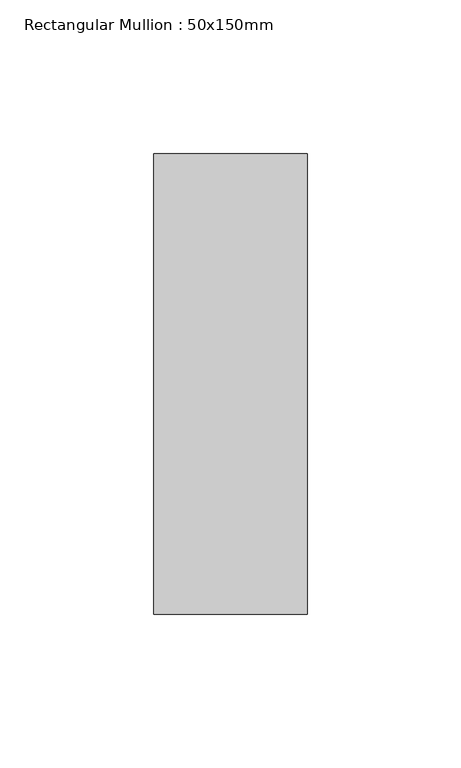
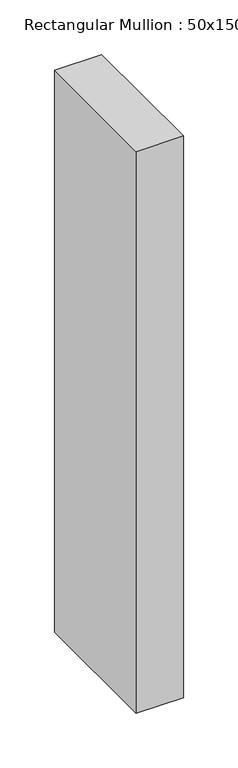
"""IFC4 building model written with IfcOpenShell, lengths in millimetres: member geometry, Rectangular Mullion : 50x150mm."""

from ifc_helpers import new_model, si_unit, frame, origin, place, context, project, spatial, polyline, outline, extrude, source, transform, mapped, element, save


def rectangular_mullion_50x150mm_ded1ff81(model_context):
    return source(origin(), model_context, "Body", "SweptSolid", [
        extrude(outline(polyline([(0.0, 75.0), (0.0, -75.0), (-50.0, -75.0), (-50.0, 75.0), (0.0, 75.0)])), frame((0.0, 0.0, -628.65), z_axis=(0.0, 0.0, 1.0), x_axis=(1.0, 0.0, 0.0)), (0.0, 0.0, 1.0), 628.65),
    ])


if __name__ == "__main__":
    model = new_model("IFC4")
    model_context = context("Model", 3, world=origin())
    ifc_project = project(units=[si_unit("LENGTHUNIT", "METRE", prefix="MILLI")], contexts=[model_context])
    site = spatial("IfcSite", under=ifc_project)
    building = spatial("IfcBuilding", under=site)
    placement = place(None, origin())
    rectangular_mullion_50x150mm_shape = rectangular_mullion_50x150mm_ded1ff81(model_context)
    element("IfcMember", 1, ObjectType="Rectangular Mullion : 50x150mm", at=placement, inside=building, context=model_context, shape_type="MappedRepresentation", body=[
        mapped(rectangular_mullion_50x150mm_shape, transform((0.0, 0.0, 0.0), x_axis=(1.0, 0.0, 0.0), y_axis=(0.0, 1.0, 0.0), z_axis=(0.0, 0.0, 1.0))),
    ])
    save(model, "model.ifc")

# Revit data of these elements
# Type "Rectangular Mullion : 50x150mm"
#   Keynote = "H11"
#   built-in parameter 1007304 = 0.492126 (stored number, unit not read)
#   built-in parameter 1007301 = 0.082021 (stored number, unit not read)
#   built-in parameter 1007300 = 0.082021 (stored number, unit not read)
# Element 1 (IfcMember, "Rectangular Mullion : 50x150mm")
#   Materials on its faces: "Aluminium"
# Materials
#   "Aluminium": class "Metal", colour RGB 247 247 247, transparency 0, Description = "Aluminium 6061", Cost = 0
